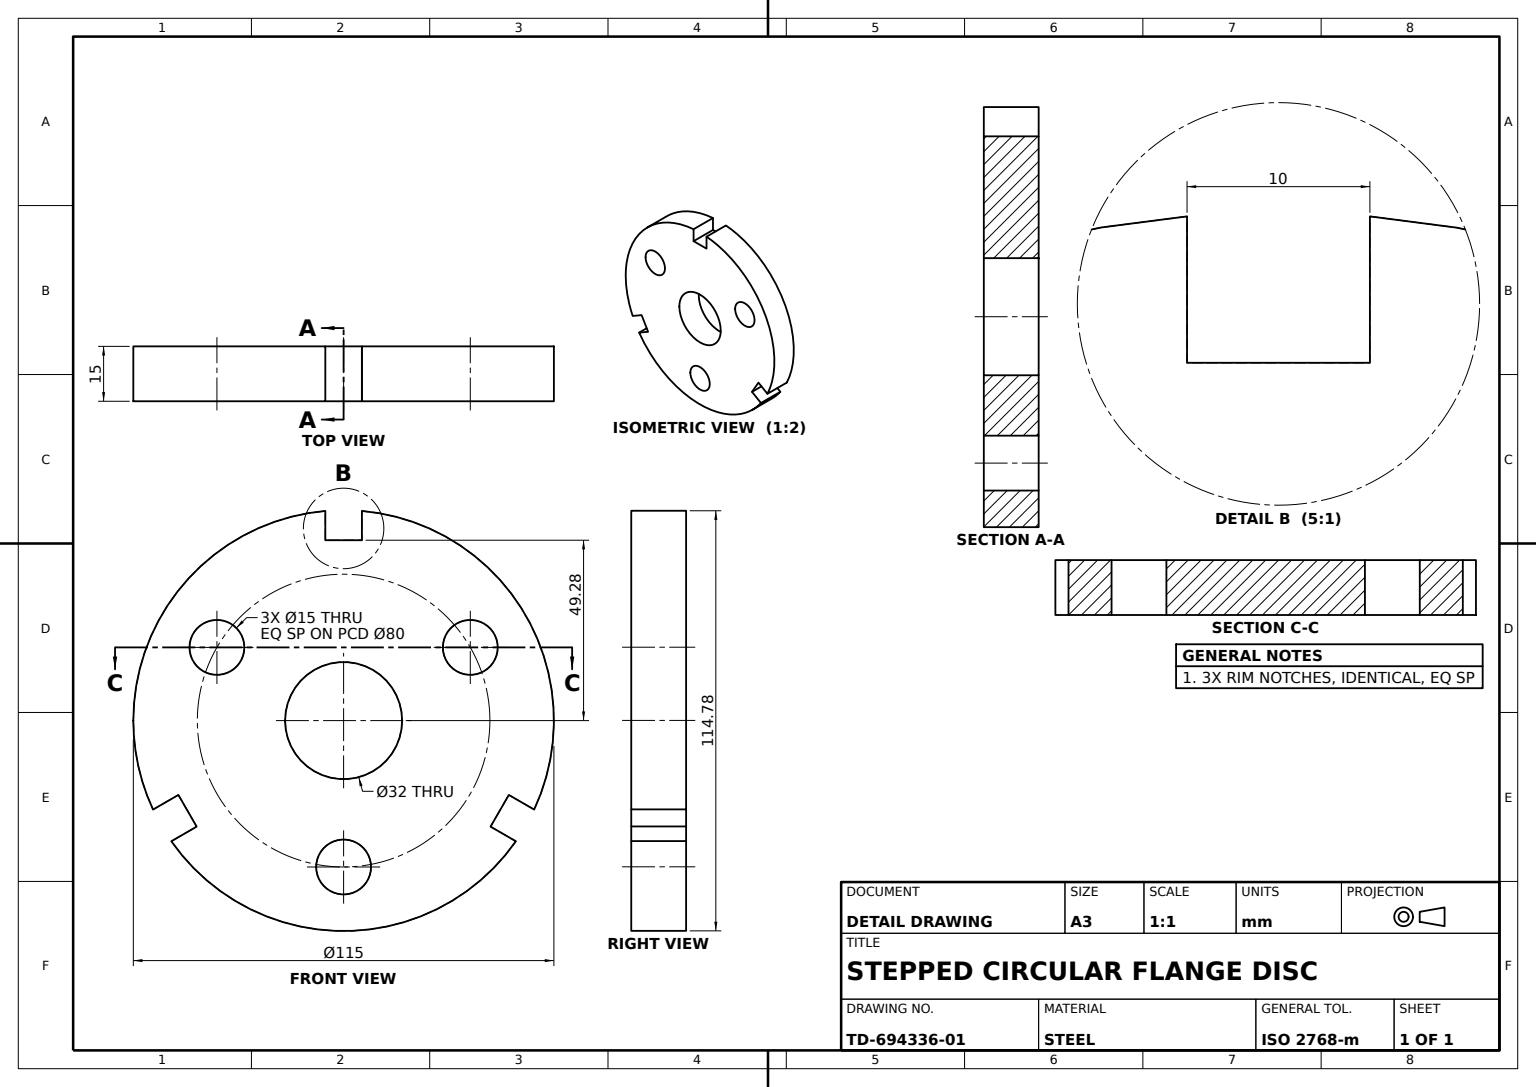
from build123d import *

# Parameters (mm, degrees)
DISC_PROFILE_115_R      = 57.5
DISC_115X15_DEPTH       = 15
HOLES_4X_15_SKETCH_R    = 7.5
HOLES_4X_15_ON_80_DEPTH = 15
CENTRE_BORE_32_SKETCH_R = 16
CENTRE_BORE_32_DEPTH    = 15
RIM_START               = -15
RIM_NOTCHES_DEPTH       = 15


with BuildPart() as part:
    # Disc Profile Ø115 → Disc Ø115x15 (new body)
    with BuildSketch(Plane.XY):
        Circle(DISC_PROFILE_115_R)
    extrude(amount=DISC_115X15_DEPTH)

    # Holes 4xØ15 Sketch → Holes 4xØ15 on Ø80 (cut)
    with BuildSketch(Plane.XY.offset(15)):
        with Locations((34.641016151, 20)):
            Circle(HOLES_4X_15_SKETCH_R)
        with Locations((0, -40)):
            Circle(HOLES_4X_15_SKETCH_R)
        with Locations((-34.641016151, 20)):
            Circle(HOLES_4X_15_SKETCH_R)
    extrude(amount=-HOLES_4X_15_ON_80_DEPTH, mode=Mode.SUBTRACT)

    # Centre Bore Ø32 Sketch → Centre Bore Ø32 (cut)
    with BuildSketch(Plane.XY.offset(15)):
        Circle(CENTRE_BORE_32_SKETCH_R)
    extrude(amount=-CENTRE_BORE_32_DEPTH, mode=Mode.SUBTRACT)

    # Rim Notches Sketch → Rim Notches (cut)
    with BuildSketch(Plane.XY.offset(15).offset(RIM_START)):
        with BuildLine():
            Line((-5, 49.282196187), (5, 49.282196187))
            Line((5, 49.282196187), (5, 57.282196187))
            ThreePointArc((5, 57.282196187), (0, 57.5), (-5, 57.282196187))
            Line((-5, 57.282196187), (-5, 49.282196187))
        make_face()
        with BuildLine():
            Line((45.179633852, -20.310971075), (40.179633852, -28.971225112))
            Line((40.179633852, -28.971225112), (47.107837082, -32.971225112))
            ThreePointArc((47.107837082, -32.971225112), (49.796460718, -28.75), (52.107837082, -24.310971075))
            Line((52.107837082, -24.310971075), (45.179633852, -20.310971075))
        make_face()
        with BuildLine():
            Line((-40.179633852, -28.971225112), (-45.179633852, -20.310971075))
            Line((-45.179633852, -20.310971075), (-52.107837082, -24.310971075))
            ThreePointArc((-52.107837082, -24.310971075), (-49.796460718, -28.75), (-47.107837082, -32.971225112))
            Line((-47.107837082, -32.971225112), (-40.179633852, -28.971225112))
        make_face()
    extrude(amount=RIM_NOTCHES_DEPTH, mode=Mode.SUBTRACT)


solid = part.part
